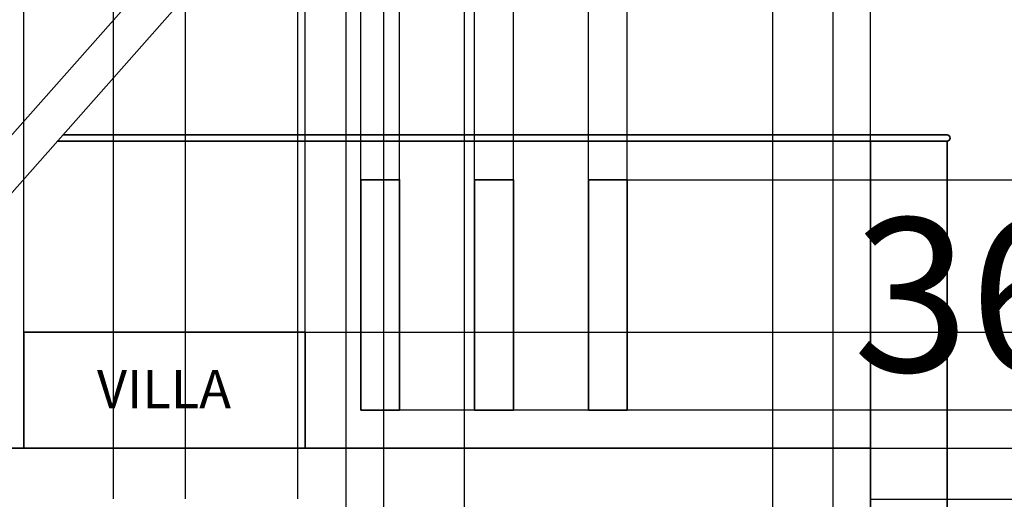
# Model space of a CAD drawing. Units: inches. Extents: x 172 to 828, y 190 to 777.
# Tile 6 of 9: x 474 to 628, y 607 to 682. Entities that reach past the tile are written whole.
import ezdxf

# ---------------------------------------------------------------- set-up
doc = ezdxf.new("R2010")
doc.units = ezdxf.units.IN
doc.header["$MEASUREMENT"] = 0
for name, color, linetype, lineweight in [('A-ANNO-DIMS', 2, 'Continuous', 18), ('A-ANNO-TEXT', 7, 'Continuous', 25), ('A-ELEV', 7, 'Continuous', 35)]:
    doc.layers.add(name, color=color, linetype=linetype, lineweight=lineweight)
doc.styles.get("Standard").update_dxf_attribs({"font": 'arial.ttf'})
doc.dimstyles.get("Standard").update_dxf_attribs({"dimtxt": 24, "dimasz": 12, "dimexe": 0.18, "dimexo": 0.0625, "dimgap": 0.09, "dimtad": 0, "dimtih": 1, "dimtoh": 1, "dimdec": 0, "dimzin": 0, "dimdsep": 46, "dimlunit": 3, "dimtxsty": 'Standard', "dimcen": 0.09, "dimadec": 0, "dimazin": 0, "dimtfac": 1, "dimtdec": 0, "dimtofl": 0, "dimtmove": 0, "dimatfit": 3, "dimfxl": 1, "dimtolj": 1, "dimtzin": 0, "dimarcsym": 0})

# ---------------------------------------------------------------- blocks, each defined once
blk = doc.blocks.new('*D6')
at = {"layer": 'A-ANNO-DIMS', "color": 0, "lineweight": -2, "transparency": 16777216}
for p, q in [((411.3, 579.39), (424.02, 579.39)), ((423.84, 567.39), (423.84, 549.9)), ((423.84, 507.39), (423.84, 524.88)), ((411.3, 495.39), (424.02, 495.39))]:
    blk.add_line(p, q, dxfattribs=at)
at = {"layer": 'A-ANNO-DIMS', "color": 0, "transparency": 16777216}
for points in [[(421.84, 567.39), (425.84, 567.39), (423.84, 579.39)], [(421.84, 507.39), (425.84, 507.39), (423.84, 495.39)]]:
    blk.add_solid(points, dxfattribs=at)
at = {"layer": 'Defpoints', "color": 0, "transparency": 16777216}
for p in [(411.24, 579.39), (423.84, 579.39), (411.24, 495.39)]:
    blk.add_point(p, dxfattribs=at)
at = {"layer": 'A-ANNO-DIMS', "color": 0, "transparency": 16777216, "insert": (423.84, 537.39), "char_height": 24, "attachment_point": 5}
blk.add_mtext('\\A1;GLAZED DOUBLE DOOR 84 TYP.', dxfattribs=at)
blk = doc.blocks.new('*D10')
at = {"layer": 'A-ANNO-DIMS', "color": 0, "lineweight": -2, "transparency": 16777216}
for p, q in [((258.78, 231.45), (258.78, 761.27)), ((270.78, 761.09), (412.23, 761.09)), ((606.78, 761.09), (465.33, 761.09)), ((618.78, 735.45), (618.78, 761.27))]:
    blk.add_line(p, q, dxfattribs=at)
at = {"layer": 'A-ANNO-DIMS', "color": 0, "transparency": 16777216}
for points in [[(270.78, 763.09), (270.78, 759.09), (258.78, 761.09)], [(606.78, 763.09), (606.78, 759.09), (618.78, 761.09)]]:
    blk.add_solid(points, dxfattribs=at)
at = {"layer": 'Defpoints', "color": 0, "transparency": 16777216}
for p in [(618.78, 761.09), (618.78, 735.39), (258.78, 231.39)]:
    blk.add_point(p, dxfattribs=at)
at = {"layer": 'A-ANNO-DIMS', "color": 0, "transparency": 16777216, "insert": (438.78, 761.09), "char_height": 24, "attachment_point": 5}
blk.add_mtext('\\A1;360', dxfattribs=at)
blk = doc.blocks.new('*D11')
at = {"layer": 'A-ANNO-DIMS', "color": 0, "lineweight": -2, "transparency": 16777216}
for p, q in [((618.84, 735.39), (645.16, 735.39)), ((644.98, 723.39), (644.98, 495.74)), ((644.98, 243.39), (644.98, 471.05)), ((618.84, 231.39), (645.16, 231.39))]:
    blk.add_line(p, q, dxfattribs=at)
at = {"layer": 'A-ANNO-DIMS', "color": 0, "transparency": 16777216}
for points in [[(642.98, 723.39), (646.98, 723.39), (644.98, 735.39)], [(642.98, 243.39), (646.98, 243.39), (644.98, 231.39)]]:
    blk.add_solid(points, dxfattribs=at)
at = {"layer": 'Defpoints', "color": 0, "transparency": 16777216}
for p in [(618.78, 735.39), (644.98, 735.39), (618.78, 231.39)]:
    blk.add_point(p, dxfattribs=at)
at = {"layer": 'A-ANNO-DIMS', "color": 0, "transparency": 16777216, "insert": (644.98, 483.39), "char_height": 24, "attachment_point": 5}
blk.add_mtext('\\A1;504', dxfattribs=at)
blk = doc.blocks.new('*D45')
at = {"layer": 'A-ANNO-DIMS', "color": 0, "lineweight": -2, "transparency": 16777216}
for p, q in [((389.1, 727.47), (389.1, 761.27)), ((401.1, 761.09), (417.14, 761.09)), ((429.14, 615.45), (429.14, 761.27)), ((429.14, 761.09), (441.14, 761.09))]:
    blk.add_line(p, q, dxfattribs=at)
at = {"layer": 'A-ANNO-DIMS', "color": 0, "transparency": 16777216}
for points in [[(401.1, 763.09), (401.1, 759.09), (389.1, 761.09)], [(417.14, 763.09), (417.14, 759.09), (429.14, 761.09)]]:
    blk.add_solid(points, dxfattribs=at)
at = {"layer": 'Defpoints', "color": 0, "transparency": 16777216}
for p in [(429.14, 761.09), (389.1, 727.4), (429.14, 615.39)]:
    blk.add_point(p, dxfattribs=at)
at = {"layer": 'A-ANNO-DIMS', "color": 0, "transparency": 16777216, "insert": (482.2, 761.09), "char_height": 24, "attachment_point": 5}
blk.add_mtext('\\A1;40.03', dxfattribs=at)
blk = doc.blocks.new('*D46')
at = {"layer": 'A-ANNO-DIMS', "color": 0, "lineweight": -2, "transparency": 16777216}
for p, q in [((429.14, 615.45), (429.14, 761.27)), ((441.14, 761.09), (445.77, 761.09)), ((485.14, 761.09), (480.51, 761.09)), ((497.14, 727.47), (497.14, 761.27))]:
    blk.add_line(p, q, dxfattribs=at)
at = {"layer": 'A-ANNO-DIMS', "color": 0, "transparency": 16777216}
for points in [[(441.14, 763.09), (441.14, 759.09), (429.14, 761.09)], [(485.14, 763.09), (485.14, 759.09), (497.14, 761.09)]]:
    blk.add_solid(points, dxfattribs=at)
at = {"layer": 'Defpoints', "color": 0, "transparency": 16777216}
for p in [(497.14, 761.09), (497.14, 727.4), (429.14, 615.39)]:
    blk.add_point(p, dxfattribs=at)
at = {"layer": 'A-ANNO-DIMS', "color": 0, "transparency": 16777216, "insert": (463.14, 761.09), "char_height": 24, "attachment_point": 5}
blk.add_mtext('\\A1;68', dxfattribs=at)
blk = doc.blocks.new('*D52')
at = {"layer": 'A-ANNO-DIMS', "color": 0, "lineweight": -2, "transparency": 16777216}
for p, q in [((409.12, 761.09), (397.12, 761.09)), ((421.12, 615.45), (421.12, 761.27)), ((429.14, 615.45), (429.14, 761.27)), ((441.14, 761.09), (453.14, 761.09))]:
    blk.add_line(p, q, dxfattribs=at)
at = {"layer": 'A-ANNO-DIMS', "color": 0, "transparency": 16777216}
for points in [[(409.12, 763.09), (409.12, 759.09), (421.12, 761.09)], [(441.14, 763.09), (441.14, 759.09), (429.14, 761.09)]]:
    blk.add_solid(points, dxfattribs=at)
at = {"layer": 'Defpoints', "color": 0, "transparency": 16777216}
for p in [(429.14, 761.09), (421.12, 615.39), (429.14, 615.39)]:
    blk.add_point(p, dxfattribs=at)
at = {"layer": 'A-ANNO-DIMS', "color": 0, "transparency": 16777216, "insert": (493.74, 761.09), "char_height": 24, "attachment_point": 5}
blk.add_mtext('\\A1;8.013', dxfattribs=at)
blk = doc.blocks.new('*D53')
at = {"layer": 'A-ANNO-DIMS', "color": 0, "lineweight": -2, "transparency": 16777216}
for p, q in [((417.14, 761.09), (405.14, 761.09)), ((429.14, 615.45), (429.14, 761.27)), ((437.15, 615.45), (437.15, 761.27)), ((449.15, 761.09), (461.15, 761.09))]:
    blk.add_line(p, q, dxfattribs=at)
at = {"layer": 'A-ANNO-DIMS', "color": 0, "transparency": 16777216}
for points in [[(417.14, 763.09), (417.14, 759.09), (429.14, 761.09)], [(449.15, 763.09), (449.15, 759.09), (437.15, 761.09)]]:
    blk.add_solid(points, dxfattribs=at)
at = {"layer": 'Defpoints', "color": 0, "transparency": 16777216}
for p in [(437.15, 761.09), (429.14, 615.39), (437.15, 615.39)]:
    blk.add_point(p, dxfattribs=at)
at = {"layer": 'A-ANNO-DIMS', "color": 0, "transparency": 16777216, "insert": (501.75, 761.09), "char_height": 24, "attachment_point": 5}
blk.add_mtext('\\A1;8.013', dxfattribs=at)
blk = doc.blocks.new('*D54')
at = {"layer": 'A-ANNO-DIMS', "color": 0, "lineweight": -2, "transparency": 16777216}
for p, q in [((267.48, 615.45), (267.48, 761.27)), ((279.48, 761.09), (330.13, 761.09)), ((462.39, 761.09), (411.75, 761.09)), ((474.39, 633.61), (474.39, 761.27))]:
    blk.add_line(p, q, dxfattribs=at)
at = {"layer": 'A-ANNO-DIMS', "color": 0, "transparency": 16777216}
for points in [[(279.48, 763.09), (279.48, 759.09), (267.48, 761.09)], [(462.39, 763.09), (462.39, 759.09), (474.39, 761.09)]]:
    blk.add_solid(points, dxfattribs=at)
at = {"layer": 'Defpoints', "color": 0, "transparency": 16777216}
for p in [(474.39, 761.09), (474.39, 633.55), (267.48, 615.39)]:
    blk.add_point(p, dxfattribs=at)
at = {"layer": 'A-ANNO-DIMS', "color": 0, "transparency": 16777216, "insert": (370.94, 761.09), "char_height": 24, "attachment_point": 5}
blk.add_mtext('\\A1;206.9', dxfattribs=at)
blk = doc.blocks.new('*D55')
at = {"layer": 'A-ANNO-DIMS', "color": 0, "lineweight": -2, "transparency": 16777216}
for p, q in [((474.39, 633.61), (474.39, 761.27)), ((486.39, 761.09), (506.4, 761.09)), ((518.4, 633.61), (518.4, 761.27)), ((518.4, 761.09), (530.4, 761.09))]:
    blk.add_line(p, q, dxfattribs=at)
at = {"layer": 'A-ANNO-DIMS', "color": 0, "transparency": 16777216}
for points in [[(486.39, 763.09), (486.39, 759.09), (474.39, 761.09)], [(506.4, 763.09), (506.4, 759.09), (518.4, 761.09)]]:
    blk.add_solid(points, dxfattribs=at)
at = {"layer": 'Defpoints', "color": 0, "transparency": 16777216}
for p in [(518.4, 761.09), (474.39, 633.55), (518.4, 633.55)]:
    blk.add_point(p, dxfattribs=at)
at = {"layer": 'A-ANNO-DIMS', "color": 0, "transparency": 16777216, "insert": (569.15, 761.09), "char_height": 24, "attachment_point": 5}
blk.add_mtext('\\A1;44.01', dxfattribs=at)
blk = doc.blocks.new('*D56')
at = {"layer": 'A-ANNO-DIMS', "color": 0, "lineweight": -2, "transparency": 16777216}
for p, q in [((506.4, 761.09), (494.4, 761.09)), ((518.4, 633.61), (518.4, 761.27)), ((527.09, 657.43), (527.09, 761.27)), ((539.09, 761.09), (551.09, 761.09))]:
    blk.add_line(p, q, dxfattribs=at)
at = {"layer": 'A-ANNO-DIMS', "color": 0, "transparency": 16777216}
for points in [[(506.4, 763.09), (506.4, 759.09), (518.4, 761.09)], [(539.09, 763.09), (539.09, 759.09), (527.09, 761.09)]]:
    blk.add_solid(points, dxfattribs=at)
at = {"layer": 'Defpoints', "color": 0, "transparency": 16777216}
for p in [(527.09, 761.09), (527.09, 657.37), (518.4, 633.55)]:
    blk.add_point(p, dxfattribs=at)
at = {"layer": 'A-ANNO-DIMS', "color": 0, "transparency": 16777216, "insert": (582.4, 761.09), "char_height": 24, "attachment_point": 5}
blk.add_mtext('\\A1;8.69', dxfattribs=at)
blk = doc.blocks.new('*D57')
at = {"layer": 'A-ANNO-DIMS', "color": 0, "lineweight": -2, "transparency": 16777216}
for p, q in [((515.09, 761.09), (503.09, 761.09)), ((527.09, 657.43), (527.09, 761.27)), ((533.17, 657.43), (533.17, 761.27)), ((545.17, 761.09), (557.17, 761.09))]:
    blk.add_line(p, q, dxfattribs=at)
at = {"layer": 'A-ANNO-DIMS', "color": 0, "transparency": 16777216}
for points in [[(515.09, 763.09), (515.09, 759.09), (527.09, 761.09)], [(545.17, 763.09), (545.17, 759.09), (533.17, 761.09)]]:
    blk.add_solid(points, dxfattribs=at)
at = {"layer": 'Defpoints', "color": 0, "transparency": 16777216}
for p in [(533.17, 761.09), (527.09, 657.37), (533.17, 657.37)]:
    blk.add_point(p, dxfattribs=at)
at = {"layer": 'A-ANNO-DIMS', "color": 0, "transparency": 16777216, "insert": (597.85, 761.09), "char_height": 24, "attachment_point": 5}
blk.add_mtext('\\A1;6.078', dxfattribs=at)
blk = doc.blocks.new('*D58')
at = {"layer": 'A-ANNO-DIMS', "color": 0, "lineweight": -2, "transparency": 16777216}
for p, q in [((521.17, 761.09), (509.17, 761.09)), ((533.17, 657.43), (533.17, 761.27)), ((544.89, 657.43), (544.89, 761.27)), ((556.89, 761.09), (568.89, 761.09))]:
    blk.add_line(p, q, dxfattribs=at)
at = {"layer": 'A-ANNO-DIMS', "color": 0, "transparency": 16777216}
for points in [[(521.17, 763.09), (521.17, 759.09), (533.17, 761.09)], [(556.89, 763.09), (556.89, 759.09), (544.89, 761.09)]]:
    blk.add_solid(points, dxfattribs=at)
at = {"layer": 'Defpoints', "color": 0, "transparency": 16777216}
for p in [(544.89, 761.09), (533.17, 657.37), (544.89, 657.37)]:
    blk.add_point(p, dxfattribs=at)
at = {"layer": 'A-ANNO-DIMS', "color": 0, "transparency": 16777216, "insert": (608.22, 761.09), "char_height": 24, "attachment_point": 5}
blk.add_mtext('\\A1;11.72', dxfattribs=at)
blk = doc.blocks.new('*D59')
at = {"layer": 'A-ANNO-DIMS', "color": 0, "lineweight": -2, "transparency": 16777216}
for p, q in [((532.89, 761.09), (520.89, 761.09)), ((544.89, 657.43), (544.89, 761.27)), ((550.97, 657.43), (550.97, 761.27)), ((562.97, 761.09), (574.97, 761.09))]:
    blk.add_line(p, q, dxfattribs=at)
at = {"layer": 'A-ANNO-DIMS', "color": 0, "transparency": 16777216}
for points in [[(532.89, 763.09), (532.89, 759.09), (544.89, 761.09)], [(562.97, 763.09), (562.97, 759.09), (550.97, 761.09)]]:
    blk.add_solid(points, dxfattribs=at)
at = {"layer": 'Defpoints', "color": 0, "transparency": 16777216}
for p in [(550.97, 761.09), (544.89, 657.37), (550.97, 657.37)]:
    blk.add_point(p, dxfattribs=at)
at = {"layer": 'A-ANNO-DIMS', "color": 0, "transparency": 16777216, "insert": (615.64, 761.09), "char_height": 24, "attachment_point": 5}
blk.add_mtext('\\A1;6.078', dxfattribs=at)
blk = doc.blocks.new('*D60')
at = {"layer": 'A-ANNO-DIMS', "color": 0, "lineweight": -2, "transparency": 16777216}
for p, q in [((538.97, 761.09), (526.97, 761.09)), ((550.97, 657.43), (550.97, 761.27)), ((562.69, 657.43), (562.69, 761.27)), ((574.69, 761.09), (586.69, 761.09))]:
    blk.add_line(p, q, dxfattribs=at)
at = {"layer": 'A-ANNO-DIMS', "color": 0, "transparency": 16777216}
for points in [[(538.97, 763.09), (538.97, 759.09), (550.97, 761.09)], [(574.69, 763.09), (574.69, 759.09), (562.69, 761.09)]]:
    blk.add_solid(points, dxfattribs=at)
at = {"layer": 'Defpoints', "color": 0, "transparency": 16777216}
for p in [(562.69, 761.09), (550.97, 657.37), (562.69, 657.37)]:
    blk.add_point(p, dxfattribs=at)
at = {"layer": 'A-ANNO-DIMS', "color": 0, "transparency": 16777216, "insert": (626.02, 761.09), "char_height": 24, "attachment_point": 5}
blk.add_mtext('\\A1;11.72', dxfattribs=at)
blk = doc.blocks.new('*D61')
at = {"layer": 'A-ANNO-DIMS', "color": 0, "lineweight": -2, "transparency": 16777216}
for p, q in [((550.69, 761.09), (538.69, 761.09)), ((562.69, 657.43), (562.69, 761.27)), ((568.77, 657.43), (568.77, 761.27)), ((580.77, 761.09), (592.77, 761.09))]:
    blk.add_line(p, q, dxfattribs=at)
at = {"layer": 'A-ANNO-DIMS', "color": 0, "transparency": 16777216}
for points in [[(550.69, 763.09), (550.69, 759.09), (562.69, 761.09)], [(580.77, 763.09), (580.77, 759.09), (568.77, 761.09)]]:
    blk.add_solid(points, dxfattribs=at)
at = {"layer": 'Defpoints', "color": 0, "transparency": 16777216}
for p in [(568.77, 761.09), (562.69, 657.37), (568.77, 657.37)]:
    blk.add_point(p, dxfattribs=at)
at = {"layer": 'A-ANNO-DIMS', "color": 0, "transparency": 16777216, "insert": (633.44, 761.09), "char_height": 24, "attachment_point": 5}
blk.add_mtext('\\A1;6.078', dxfattribs=at)
blk = doc.blocks.new('*D62')
at = {"layer": 'A-ANNO-DIMS', "color": 0, "lineweight": -2, "transparency": 16777216}
for p, q in [((568.77, 657.43), (568.77, 761.27)), ((580.77, 761.09), (594.82, 761.09)), ((606.82, 663.45), (606.82, 761.27)), ((606.82, 761.09), (618.82, 761.09))]:
    blk.add_line(p, q, dxfattribs=at)
at = {"layer": 'A-ANNO-DIMS', "color": 0, "transparency": 16777216}
for points in [[(580.77, 763.09), (580.77, 759.09), (568.77, 761.09)], [(594.82, 763.09), (594.82, 759.09), (606.82, 761.09)]]:
    blk.add_solid(points, dxfattribs=at)
at = {"layer": 'Defpoints', "color": 0, "transparency": 16777216}
for p in [(606.82, 761.09), (606.82, 663.39), (568.77, 657.37)]:
    blk.add_point(p, dxfattribs=at)
at = {"layer": 'A-ANNO-DIMS', "color": 0, "transparency": 16777216, "insert": (659.48, 761.09), "char_height": 24, "attachment_point": 5}
blk.add_mtext('\\A1;38.05', dxfattribs=at)
blk = doc.blocks.new('*D63')
at = {"layer": 'A-ANNO-DIMS', "color": 0, "lineweight": -2, "transparency": 16777216}
for p, q in [((594.82, 761.09), (582.82, 761.09)), ((606.82, 663.45), (606.82, 761.27)), ((618.78, 723.23), (618.78, 761.27)), ((630.78, 761.09), (642.78, 761.09))]:
    blk.add_line(p, q, dxfattribs=at)
at = {"layer": 'A-ANNO-DIMS', "color": 0, "transparency": 16777216}
for points in [[(594.82, 763.09), (594.82, 759.09), (606.82, 761.09)], [(630.78, 763.09), (630.78, 759.09), (618.78, 761.09)]]:
    blk.add_solid(points, dxfattribs=at)
at = {"layer": 'Defpoints', "color": 0, "transparency": 16777216}
for p in [(618.78, 761.09), (618.78, 723.17), (606.82, 663.39)]:
    blk.add_point(p, dxfattribs=at)
at = {"layer": 'A-ANNO-DIMS', "color": 0, "transparency": 16777216, "insert": (691.56, 761.09), "char_height": 24, "attachment_point": 5}
blk.add_mtext('\\A1;11.963', dxfattribs=at)
blk = doc.blocks.new('*D64')
at = {"layer": 'A-ANNO-DIMS', "color": 0, "lineweight": -2, "transparency": 16777216}
for p, q in [((644.98, 645.55), (644.98, 657.55)), ((644.98, 657.55), (656.98, 657.55)), ((518.47, 633.55), (645.16, 633.55)), ((518.47, 615.39), (645.16, 615.39)), ((644.98, 603.39), (644.98, 591.39))]:
    blk.add_line(p, q, dxfattribs=at)
at = {"layer": 'A-ANNO-DIMS', "color": 0, "transparency": 16777216}
for points in [[(642.98, 645.55), (646.98, 645.55), (644.98, 633.55)], [(642.98, 603.39), (646.98, 603.39), (644.98, 615.39)]]:
    blk.add_solid(points, dxfattribs=at)
at = {"layer": 'Defpoints', "color": 0, "transparency": 16777216}
for p in [(518.4, 633.55), (644.98, 633.55), (518.4, 615.39)]:
    blk.add_point(p, dxfattribs=at)
at = {"layer": 'A-ANNO-DIMS', "color": 0, "transparency": 16777216, "insert": (696.43, 657.55), "char_height": 24, "attachment_point": 5}
blk.add_mtext('\\A1;18.16', dxfattribs=at)
blk = doc.blocks.new('*D65')
at = {"layer": 'A-ANNO-DIMS', "color": 0, "lineweight": -2, "transparency": 16777216}
for p, q in [((644.98, 633.36), (644.98, 645.36)), ((644.98, 645.36), (656.98, 645.36)), ((527.16, 621.36), (645.16, 621.36)), ((518.47, 615.39), (645.16, 615.39)), ((644.98, 603.39), (644.98, 591.39))]:
    blk.add_line(p, q, dxfattribs=at)
at = {"layer": 'A-ANNO-DIMS', "color": 0, "transparency": 16777216}
for points in [[(642.98, 633.36), (646.98, 633.36), (644.98, 621.36)], [(642.98, 603.39), (646.98, 603.39), (644.98, 615.39)]]:
    blk.add_solid(points, dxfattribs=at)
at = {"layer": 'Defpoints', "color": 0, "transparency": 16777216}
for p in [(527.09, 621.36), (644.98, 621.36), (518.4, 615.39)]:
    blk.add_point(p, dxfattribs=at)
at = {"layer": 'A-ANNO-DIMS', "color": 0, "transparency": 16777216, "insert": (697.55, 645.36), "char_height": 24, "attachment_point": 5}
blk.add_mtext('\\A1;5.966', dxfattribs=at)
blk = doc.blocks.new('*D66')
at = {"layer": 'A-ANNO-DIMS', "color": 0, "lineweight": -2, "transparency": 16777216}
for p, q in [((644.98, 669.37), (644.98, 681.37)), ((568.83, 657.37), (645.16, 657.37)), ((568.83, 621.36), (645.16, 621.36)), ((644.98, 609.36), (644.98, 597.36))]:
    blk.add_line(p, q, dxfattribs=at)
at = {"layer": 'A-ANNO-DIMS', "color": 0, "transparency": 16777216}
for points in [[(642.98, 669.37), (646.98, 669.37), (644.98, 657.37)], [(642.98, 609.36), (646.98, 609.36), (644.98, 621.36)]]:
    blk.add_solid(points, dxfattribs=at)
at = {"layer": 'Defpoints', "color": 0, "transparency": 16777216}
for p in [(568.77, 657.37), (644.98, 657.37), (568.77, 621.36)]:
    blk.add_point(p, dxfattribs=at)
at = {"layer": 'A-ANNO-DIMS', "color": 0, "transparency": 16777216, "insert": (644.98, 639.36), "char_height": 24, "attachment_point": 5}
blk.add_mtext('\\A1;36.01', dxfattribs=at)
blk = doc.blocks.new('*D76')
at = {"layer": 'A-ANNO-DIMS', "color": 0, "lineweight": -2, "transparency": 16777216}
for p, q in [((399.24, 761.09), (387.24, 761.09)), ((411.24, 495.45), (411.24, 761.27)), ((427.59, 495.45), (427.59, 761.27)), ((439.59, 761.09), (451.59, 761.09))]:
    blk.add_line(p, q, dxfattribs=at)
at = {"layer": 'A-ANNO-DIMS', "color": 0, "transparency": 16777216}
for points in [[(399.24, 763.09), (399.24, 759.09), (411.24, 761.09)], [(439.59, 763.09), (439.59, 759.09), (427.59, 761.09)]]:
    blk.add_solid(points, dxfattribs=at)
at = {"layer": 'Defpoints', "color": 0, "transparency": 16777216}
for p in [(427.59, 761.09), (411.24, 495.39), (427.59, 495.39)]:
    blk.add_point(p, dxfattribs=at)
at = {"layer": 'A-ANNO-DIMS', "color": 0, "transparency": 16777216, "insert": (500.36, 761.09), "char_height": 24, "attachment_point": 5}
blk.add_mtext('\\A1;16.356', dxfattribs=at)
blk = doc.blocks.new('*D77')
at = {"layer": 'A-ANNO-DIMS', "color": 0, "lineweight": -2, "transparency": 16777216}
for p, q in [((427.59, 495.45), (427.59, 761.27)), ((439.59, 761.09), (452.34, 761.09)), ((464.34, 495.45), (464.34, 761.27)), ((464.34, 761.09), (476.34, 761.09))]:
    blk.add_line(p, q, dxfattribs=at)
at = {"layer": 'A-ANNO-DIMS', "color": 0, "transparency": 16777216}
for points in [[(439.59, 763.09), (439.59, 759.09), (427.59, 761.09)], [(452.34, 763.09), (452.34, 759.09), (464.34, 761.09)]]:
    blk.add_solid(points, dxfattribs=at)
at = {"layer": 'Defpoints', "color": 0, "transparency": 16777216}
for p in [(464.34, 761.09), (427.59, 495.39), (464.34, 495.39)]:
    blk.add_point(p, dxfattribs=at)
at = {"layer": 'A-ANNO-DIMS', "color": 0, "transparency": 16777216, "insert": (516.86, 761.09), "char_height": 24, "attachment_point": 5}
blk.add_mtext('\\A1;36.74', dxfattribs=at)
blk = doc.blocks.new('*D78')
at = {"layer": 'A-ANNO-DIMS', "color": 0, "lineweight": -2, "transparency": 16777216}
for p, q in [((452.34, 761.09), (440.34, 761.09)), ((464.34, 607.45), (464.34, 761.27)), ((488.42, 607.45), (488.42, 761.27)), ((500.42, 761.09), (512.42, 761.09))]:
    blk.add_line(p, q, dxfattribs=at)
at = {"layer": 'A-ANNO-DIMS', "color": 0, "transparency": 16777216}
for points in [[(452.34, 763.09), (452.34, 759.09), (464.34, 761.09)], [(500.42, 763.09), (500.42, 759.09), (488.42, 761.09)]]:
    blk.add_solid(points, dxfattribs=at)
at = {"layer": 'Defpoints', "color": 0, "transparency": 16777216}
for p in [(488.42, 761.09), (464.34, 607.39), (488.42, 607.39)]:
    blk.add_point(p, dxfattribs=at)
at = {"layer": 'A-ANNO-DIMS', "color": 0, "transparency": 16777216, "insert": (562.56, 761.09), "char_height": 24, "attachment_point": 5}
blk.add_mtext('\\A1;24.088', dxfattribs=at)
blk = doc.blocks.new('*D79')
at = {"layer": 'A-ANNO-DIMS', "color": 0, "lineweight": -2, "transparency": 16777216}
for p, q in [((476.42, 761.09), (464.42, 761.09)), ((488.42, 607.45), (488.42, 761.27)), ((499.69, 607.45), (499.69, 761.27)), ((511.69, 761.09), (523.69, 761.09))]:
    blk.add_line(p, q, dxfattribs=at)
at = {"layer": 'A-ANNO-DIMS', "color": 0, "transparency": 16777216}
for points in [[(476.42, 763.09), (476.42, 759.09), (488.42, 761.09)], [(511.69, 763.09), (511.69, 759.09), (499.69, 761.09)]]:
    blk.add_solid(points, dxfattribs=at)
at = {"layer": 'Defpoints', "color": 0, "transparency": 16777216}
for p in [(499.69, 761.09), (488.42, 607.39), (499.69, 607.39)]:
    blk.add_point(p, dxfattribs=at)
at = {"layer": 'A-ANNO-DIMS', "color": 0, "transparency": 16777216, "insert": (563.15, 761.09), "char_height": 24, "attachment_point": 5}
blk.add_mtext('\\A1;11.27', dxfattribs=at)
blk = doc.blocks.new('*D80')
at = {"layer": 'A-ANNO-DIMS', "color": 0, "lineweight": -2, "transparency": 16777216}
for p, q in [((487.69, 761.09), (475.69, 761.09)), ((499.69, 607.45), (499.69, 761.27)), ((517.23, 607.45), (517.23, 761.27)), ((529.23, 761.09), (541.23, 761.09))]:
    blk.add_line(p, q, dxfattribs=at)
at = {"layer": 'A-ANNO-DIMS', "color": 0, "transparency": 16777216}
for points in [[(487.69, 763.09), (487.69, 759.09), (499.69, 761.09)], [(529.23, 763.09), (529.23, 759.09), (517.23, 761.09)]]:
    blk.add_solid(points, dxfattribs=at)
at = {"layer": 'Defpoints', "color": 0, "transparency": 16777216}
for p in [(517.23, 761.09), (499.69, 607.39), (517.23, 607.39)]:
    blk.add_point(p, dxfattribs=at)
at = {"layer": 'A-ANNO-DIMS', "color": 0, "transparency": 16777216, "insert": (590, 761.09), "char_height": 24, "attachment_point": 5}
blk.add_mtext('\\A1;17.533', dxfattribs=at)
blk = doc.blocks.new('*D81')
at = {"layer": 'A-ANNO-DIMS', "color": 0, "lineweight": -2, "transparency": 16777216}
for p, q in [((505.23, 761.09), (493.23, 761.09)), ((517.23, 607.45), (517.23, 761.27)), ((524.83, 493.45), (524.83, 761.27)), ((536.83, 761.09), (548.83, 761.09))]:
    blk.add_line(p, q, dxfattribs=at)
at = {"layer": 'A-ANNO-DIMS', "color": 0, "transparency": 16777216}
for points in [[(505.23, 763.09), (505.23, 759.09), (517.23, 761.09)], [(536.83, 763.09), (536.83, 759.09), (524.83, 761.09)]]:
    blk.add_solid(points, dxfattribs=at)
at = {"layer": 'Defpoints', "color": 0, "transparency": 16777216}
for p in [(524.83, 761.09), (517.23, 607.39), (524.83, 493.39)]:
    blk.add_point(p, dxfattribs=at)
at = {"layer": 'A-ANNO-DIMS', "color": 0, "transparency": 16777216, "insert": (570.66, 761.09), "char_height": 24, "attachment_point": 5}
blk.add_mtext('\\A1;7.6', dxfattribs=at)
blk = doc.blocks.new('*D82')
at = {"layer": 'A-ANNO-DIMS', "color": 0, "lineweight": -2, "transparency": 16777216}
for p, q in [((588.96, 761.09), (576.96, 761.09)), ((600.96, 493.45), (600.96, 761.27)), ((606.82, 607.45), (606.82, 761.27)), ((618.82, 761.09), (630.82, 761.09))]:
    blk.add_line(p, q, dxfattribs=at)
at = {"layer": 'A-ANNO-DIMS', "color": 0, "transparency": 16777216}
for points in [[(588.96, 763.09), (588.96, 759.09), (600.96, 761.09)], [(618.82, 763.09), (618.82, 759.09), (606.82, 761.09)]]:
    blk.add_solid(points, dxfattribs=at)
at = {"layer": 'Defpoints', "color": 0, "transparency": 16777216}
for p in [(606.82, 761.09), (606.82, 607.39), (600.96, 493.39)]:
    blk.add_point(p, dxfattribs=at)
at = {"layer": 'A-ANNO-DIMS', "color": 0, "transparency": 16777216, "insert": (671.39, 761.09), "char_height": 24, "attachment_point": 5}
blk.add_mtext('\\A1;5.856', dxfattribs=at)
blk = doc.blocks.new('*D83')
at = {"layer": 'A-ANNO-DIMS', "color": 0, "lineweight": -2, "transparency": 16777216}
for p, q in [((512.83, 761.09), (500.83, 761.09)), ((524.83, 535.45), (524.83, 761.27)), ((543.3, 599.86), (543.3, 761.27)), ((555.3, 761.09), (567.3, 761.09))]:
    blk.add_line(p, q, dxfattribs=at)
at = {"layer": 'A-ANNO-DIMS', "color": 0, "transparency": 16777216}
for points in [[(512.83, 763.09), (512.83, 759.09), (524.83, 761.09)], [(555.3, 763.09), (555.3, 759.09), (543.3, 761.09)]]:
    blk.add_solid(points, dxfattribs=at)
at = {"layer": 'Defpoints', "color": 0, "transparency": 16777216}
for p in [(543.3, 761.09), (543.3, 599.8), (524.83, 535.39)]:
    blk.add_point(p, dxfattribs=at)
at = {"layer": 'A-ANNO-DIMS', "color": 0, "transparency": 16777216, "insert": (606.75, 761.09), "char_height": 24, "attachment_point": 5}
blk.add_mtext('\\A1;18.47', dxfattribs=at)
blk = doc.blocks.new('*D84')
at = {"layer": 'A-ANNO-DIMS', "color": 0, "lineweight": -2, "transparency": 16777216}
for p, q in [((543.3, 599.86), (543.3, 761.27)), ((555.3, 761.09), (579.54, 761.09)), ((591.54, 599.86), (591.54, 761.27)), ((591.54, 761.09), (603.54, 761.09))]:
    blk.add_line(p, q, dxfattribs=at)
at = {"layer": 'A-ANNO-DIMS', "color": 0, "transparency": 16777216}
for points in [[(555.3, 763.09), (555.3, 759.09), (543.3, 761.09)], [(579.54, 763.09), (579.54, 759.09), (591.54, 761.09)]]:
    blk.add_solid(points, dxfattribs=at)
at = {"layer": 'Defpoints', "color": 0, "transparency": 16777216}
for p in [(591.54, 761.09), (543.3, 599.8), (591.54, 599.8)]:
    blk.add_point(p, dxfattribs=at)
at = {"layer": 'A-ANNO-DIMS', "color": 0, "transparency": 16777216, "insert": (644.7, 761.09), "char_height": 24, "attachment_point": 5}
blk.add_mtext('\\A1;48.25', dxfattribs=at)
blk = doc.blocks.new('*D85')
at = {"layer": 'A-ANNO-DIMS', "color": 0, "lineweight": -2, "transparency": 16777216}
for p, q in [((579.54, 761.09), (567.54, 761.09)), ((591.54, 599.86), (591.54, 761.27)), ((600.96, 535.45), (600.96, 761.27)), ((612.96, 761.09), (624.96, 761.09))]:
    blk.add_line(p, q, dxfattribs=at)
at = {"layer": 'A-ANNO-DIMS', "color": 0, "transparency": 16777216}
for points in [[(579.54, 763.09), (579.54, 759.09), (591.54, 761.09)], [(612.96, 763.09), (612.96, 759.09), (600.96, 761.09)]]:
    blk.add_solid(points, dxfattribs=at)
at = {"layer": 'Defpoints', "color": 0, "transparency": 16777216}
for p in [(600.96, 761.09), (591.54, 599.8), (600.96, 535.39)]:
    blk.add_point(p, dxfattribs=at)
at = {"layer": 'A-ANNO-DIMS', "color": 0, "transparency": 16777216, "insert": (665.63, 761.09), "char_height": 24, "attachment_point": 5}
blk.add_mtext('\\A1;9.415', dxfattribs=at)
blk = doc.blocks.new('*D86')
at = {"layer": 'A-ANNO-DIMS', "color": 0, "lineweight": -2, "transparency": 16777216}
for p, q in [((512.83, 761.09), (500.83, 761.09)), ((524.83, 493.45), (524.83, 761.27)), ((530.68, 493.45), (530.68, 761.27)), ((542.68, 761.09), (554.68, 761.09))]:
    blk.add_line(p, q, dxfattribs=at)
at = {"layer": 'A-ANNO-DIMS', "color": 0, "transparency": 16777216}
for points in [[(512.83, 763.09), (512.83, 759.09), (524.83, 761.09)], [(542.68, 763.09), (542.68, 759.09), (530.68, 761.09)]]:
    blk.add_solid(points, dxfattribs=at)
at = {"layer": 'Defpoints', "color": 0, "transparency": 16777216}
for p in [(530.68, 761.09), (524.83, 493.39), (530.68, 493.39)]:
    blk.add_point(p, dxfattribs=at)
at = {"layer": 'A-ANNO-DIMS', "color": 0, "transparency": 16777216, "insert": (595.26, 761.09), "char_height": 24, "attachment_point": 5}
blk.add_mtext('\\A1;5.856', dxfattribs=at)
blk = doc.blocks.new('*D91')
at = {"layer": 'A-ANNO-DIMS', "color": 0, "lineweight": -2, "transparency": 16777216}
for p, q in [((644.98, 619.39), (644.98, 631.39)), ((644.98, 631.39), (656.98, 631.39)), ((606.88, 607.39), (645.16, 607.39)), ((591.61, 599.8), (645.16, 599.8)), ((644.98, 587.8), (644.98, 575.8))]:
    blk.add_line(p, q, dxfattribs=at)
at = {"layer": 'A-ANNO-DIMS', "color": 0, "transparency": 16777216}
for points in [[(642.98, 619.39), (646.98, 619.39), (644.98, 607.39)], [(642.98, 587.8), (646.98, 587.8), (644.98, 599.8)]]:
    blk.add_solid(points, dxfattribs=at)
at = {"layer": 'Defpoints', "color": 0, "transparency": 16777216}
for p in [(606.82, 607.39), (644.98, 607.39), (591.54, 599.8)]:
    blk.add_point(p, dxfattribs=at)
at = {"layer": 'A-ANNO-DIMS', "color": 0, "transparency": 16777216, "insert": (695.15, 631.39), "char_height": 24, "attachment_point": 5}
blk.add_mtext('\\A1;7.591', dxfattribs=at)

msp = doc.modelspace()

# ---------------------------------------------------------------- linework, layer by layer
at = {"layer": 'A-ELEV'}
for p, q in [((429.1355, 615.3923), (524.5502, 723.1684)), ((437.149, 615.3923), (532.5637, 723.1684)), ((618.7792, 664.3923), (480.5289, 664.3923)), ((618.7792, 663.3923), (479.6436, 663.3923)), ((606.8158, 359.3923), (606.8158, 663.3923)), ((618.7792, 359.3923), (618.7792, 663.3923)), ((606.8158, 615.3923), (267.4822, 615.3923))]:
    msp.add_line(p, q, dxfattribs=at)
for points in [[(527.0943, 621.358), (533.1719, 621.358), (533.1719, 657.3703), (527.0943, 657.3703)], [(544.8929, 621.358), (550.9705, 621.358), (550.9705, 657.3703), (544.8929, 657.3703)], [(562.6916, 621.358), (568.7692, 621.358), (568.7692, 657.3703), (562.6916, 657.3703)], [(474.3939, 615.3923), (518.4045, 615.3923), (518.4045, 633.5521), (474.3939, 633.5521)]]:
    msp.add_lwpolyline(points, close=True, dxfattribs=at)
msp.add_arc((618.7792, 663.8923), 0.5, 270, 90, dxfattribs=at)

# ---------------------------------------------------------------- texts
at = {"layer": 'A-ANNO-TEXT'}
msp.add_text('VILLA', height=6, dxfattribs=at).set_placement((485.838, 621.6388))

# ---------------------------------------------------------------- dimensions: what is measured, and where the dimension line sits
at = {"layer": 'A-ANNO-DIMS'}
for base, p1, p2, override, picture, middle in [((618.7792, 761.0923), (258.7792, 231.3923), (618.7792, 735.3923), {"dimdec": 0, "dimlfac": 1, "dimrnd": 0, "dimzin": 0, "dimdsep": 46, "dimlunit": 2}, '*D10', (438.7792, 761.0923)), ((474.3939, 761.0923), (267.4822, 615.3923), (474.3939, 633.5521), {"dimdec": 1, "dimlfac": 1, "dimrnd": 0, "dimzin": 0, "dimdsep": 46, "dimlunit": 2}, '*D54', (370.9381, 761.0923)), ((427.5926, 761.0923), (411.2362, 495.3923), (427.5926, 495.3923), {"dimdec": 3, "dimlfac": 1, "dimrnd": 0, "dimzin": 0, "dimdsep": 46, "dimlunit": 2}, '*D76', (500.362, 761.0923)), ((429.1355, 761.0923), (389.104, 727.4027), (429.1355, 615.3923), {"dimdec": 2, "dimlfac": 1, "dimrnd": 0, "dimzin": 0, "dimdsep": 46, "dimlunit": 2}, '*D45', (482.2024, 761.0923)), ((429.1355, 761.0923), (421.1221, 615.3923), (429.1355, 615.3923), {"dimdec": 3, "dimlfac": 1, "dimrnd": 0, "dimzin": 0, "dimdsep": 46, "dimlunit": 2}, '*D52', (493.7358, 761.0923)), ((437.149, 761.09229), (429.13555, 615.39229), (437.149, 615.39229), {"dimdec": 3, "dimlfac": 1, "dimrnd": 0, "dimzin": 0, "dimdsep": 46, "dimlunit": 2}, '*D53', (501.74924, 761.09229)), ((464.3356, 761.0923), (427.5926, 495.3923), (464.3356, 495.3923), {"dimdec": 2, "dimlfac": 1, "dimrnd": 0, "dimzin": 0, "dimdsep": 46, "dimlunit": 2}, '*D77', (516.8622, 761.0923)), ((497.1421, 761.0923), (429.1355, 615.3923), (497.1421, 727.4027), {"dimdec": 0, "dimlfac": 1, "dimrnd": 0, "dimzin": 0, "dimdsep": 46, "dimlunit": 2}, '*D46', (463.1388, 761.0923)), ((488.4232, 761.0923), (464.3356, 607.3923), (488.4232, 607.3923), {"dimdec": 3, "dimlfac": 1, "dimrnd": 0, "dimzin": 0, "dimdsep": 46, "dimlunit": 2}, '*D78', (562.5596, 761.0923)), ((499.6941, 761.0923), (488.4232, 607.3923), (499.6941, 607.3923), {"dimdec": 2, "dimlfac": 1, "dimrnd": 0, "dimzin": 0, "dimdsep": 46, "dimlunit": 2}, '*D79', (563.1484, 761.0923)), ((518.4045, 761.0923), (474.3939, 633.5521), (518.4045, 633.5521), {"dimdec": 2, "dimlfac": 1, "dimrnd": 0, "dimzin": 0, "dimdsep": 46, "dimlunit": 2}, '*D55', (569.1548, 761.0923)), ((517.2267, 761.0923), (499.6941, 607.3923), (517.2267, 607.3923), {"dimdec": 3, "dimlfac": 1, "dimrnd": 0, "dimzin": 0, "dimdsep": 46, "dimlunit": 2}, '*D80', (590.0043, 761.0923)), ((524.8269, 761.0923), (517.2267, 607.3923), (524.8269, 493.3923), {"dimdec": 1, "dimlfac": 1, "dimrnd": 0, "dimzin": 0, "dimdsep": 46, "dimlunit": 2}, '*D81', (570.6577, 761.0923)), ((527.0943, 761.0923), (518.4045, 633.5521), (527.0943, 657.3703), {"dimdec": 2, "dimlfac": 1, "dimrnd": 0, "dimzin": 0, "dimdsep": 46, "dimlunit": 2}, '*D56', (582.3957, 761.0923)), ((543.2956, 761.0923), (524.8269, 535.3923), (543.2956, 599.8013), {"dimdec": 2, "dimlfac": 1, "dimrnd": 0, "dimzin": 0, "dimdsep": 46, "dimlunit": 2}, '*D83', (606.7498, 761.0923)), ((530.6832, 761.0923), (524.8269, 493.3923), (530.6832, 493.3923), {"dimdec": 3, "dimlfac": 1, "dimrnd": 0, "dimzin": 0, "dimdsep": 46, "dimlunit": 2}, '*D86', (595.2589, 761.0923)), ((533.1719, 761.0923), (527.0943, 657.3703), (533.1719, 657.3703), {"dimdec": 3, "dimlfac": 1, "dimrnd": 0, "dimzin": 0, "dimdsep": 46, "dimlunit": 2}, '*D57', (597.8458, 761.0923)), ((544.8929, 761.0923), (533.1719, 657.3703), (544.8929, 657.3703), {"dimdec": 2, "dimlfac": 1, "dimrnd": 0, "dimzin": 0, "dimdsep": 46, "dimlunit": 2}, '*D58', (608.2244, 761.0923)), ((550.9705, 761.0923), (544.8929, 657.3703), (550.9705, 657.3703), {"dimdec": 3, "dimlfac": 1, "dimrnd": 0, "dimzin": 0, "dimdsep": 46, "dimlunit": 2}, '*D59', (615.6444, 761.0923)), ((562.6916, 761.0923), (550.9705, 657.3703), (562.6916, 657.3703), {"dimdec": 2, "dimlfac": 1, "dimrnd": 0, "dimzin": 0, "dimdsep": 46, "dimlunit": 2}, '*D60', (626.023, 761.0923)), ((568.7692, 761.0923), (562.6916, 657.3703), (568.7692, 657.3703), {"dimdec": 3, "dimlfac": 1, "dimrnd": 0, "dimzin": 0, "dimdsep": 46, "dimlunit": 2}, '*D61', (633.4431, 761.0923)), ((591.5446, 761.0923), (543.2956, 599.8013), (591.5446, 599.8013), {"dimdec": 2, "dimlfac": 1, "dimrnd": 0, "dimzin": 0, "dimdsep": 46, "dimlunit": 2}, '*D84', (644.7014, 761.0923)), ((600.9594, 761.0923), (591.5446, 599.8013), (600.9594, 535.3923), {"dimdec": 3, "dimlfac": 1, "dimrnd": 0, "dimzin": 0, "dimdsep": 46, "dimlunit": 2}, '*D85', (665.6333, 761.0923)), ((606.8158, 761.0923), (568.7692, 657.3703), (606.8158, 663.3923), {"dimdec": 2, "dimlfac": 1, "dimrnd": 0, "dimzin": 0, "dimdsep": 46, "dimlunit": 2}, '*D62', (659.4815, 761.0923)), ((606.8158, 761.0923), (600.9594, 493.3923), (606.8158, 607.3923), {"dimdec": 3, "dimlfac": 1, "dimrnd": 0, "dimzin": 0, "dimdsep": 46, "dimlunit": 2}, '*D82', (671.3915, 761.0923)), ((618.7792, 761.0923), (606.8158, 663.3923), (618.7792, 723.1684), {"dimdec": 3, "dimlfac": 1, "dimrnd": 0, "dimzin": 0, "dimdsep": 46, "dimlunit": 2}, '*D63', (691.5568, 761.0923))]:
    dim = msp.add_linear_dim(base=base, p1=p1, p2=p2, dimstyle='Standard', override=override, dxfattribs=at)
    dim.commit()
    dim.dimension.update_dxf_attribs({"geometry": picture, "text_midpoint": middle})
for base, p1, p2, override, picture, middle in [((644.9792, 735.3923), (618.7792, 231.3923), (618.7792, 735.3923), {"dimdec": 0, "dimlfac": 1, "dimrnd": 0, "dimzin": 0, "dimdsep": 46, "dimlunit": 2}, '*D11', (644.9792, 483.3923)), ((644.9792, 657.3703), (568.7692, 621.358), (568.7692, 657.3703), {"dimdec": 2, "dimlfac": 1, "dimrnd": 0, "dimzin": 0, "dimdsep": 46, "dimlunit": 2}, '*D66', (644.9792, 639.3642)), ((644.9792, 633.5521), (518.4045, 615.3923), (518.4045, 633.5521), {"dimdec": 2, "dimlfac": 1, "dimrnd": 0, "dimzin": 0, "dimdsep": 46, "dimlunit": 2}, '*D64', (696.4252, 657.5521)), ((644.9792, 621.358), (518.4045, 615.3923), (527.0943, 621.358), {"dimdec": 3, "dimlfac": 1, "dimrnd": 0, "dimzin": 0, "dimdsep": 46, "dimlunit": 2}, '*D65', (697.5549, 645.358)), ((644.9792, 607.3923), (591.5446, 599.8013), (606.8158, 607.3923), {"dimdec": 3, "dimlfac": 1, "dimrnd": 0, "dimzin": 0, "dimdsep": 46, "dimlunit": 2}, '*D91', (695.1483, 631.3923))]:
    dim = msp.add_linear_dim(base=base, p1=p1, p2=p2, angle=90, dimstyle='Standard', override=override, dxfattribs=at)
    dim.commit()
    dim.dimension.update_dxf_attribs({"geometry": picture, "text_midpoint": middle})
dim = msp.add_linear_dim(base=(423.8362, 579.3923), p1=(411.2362, 495.3923), p2=(411.2362, 579.3923), angle=90, text='GLAZED DOUBLE DOOR <> TYP.', dimstyle='Standard', override={"dimdec": 0, "dimlfac": 1, "dimrnd": 0, "dimzin": 0, "dimdsep": 46, "dimlunit": 2}, dxfattribs=at)
dim.commit()
dim.dimension.update_dxf_attribs({"geometry": '*D6', "text_midpoint": (423.8362, 537.3923)})

doc.saveas('drawing.dxf')
